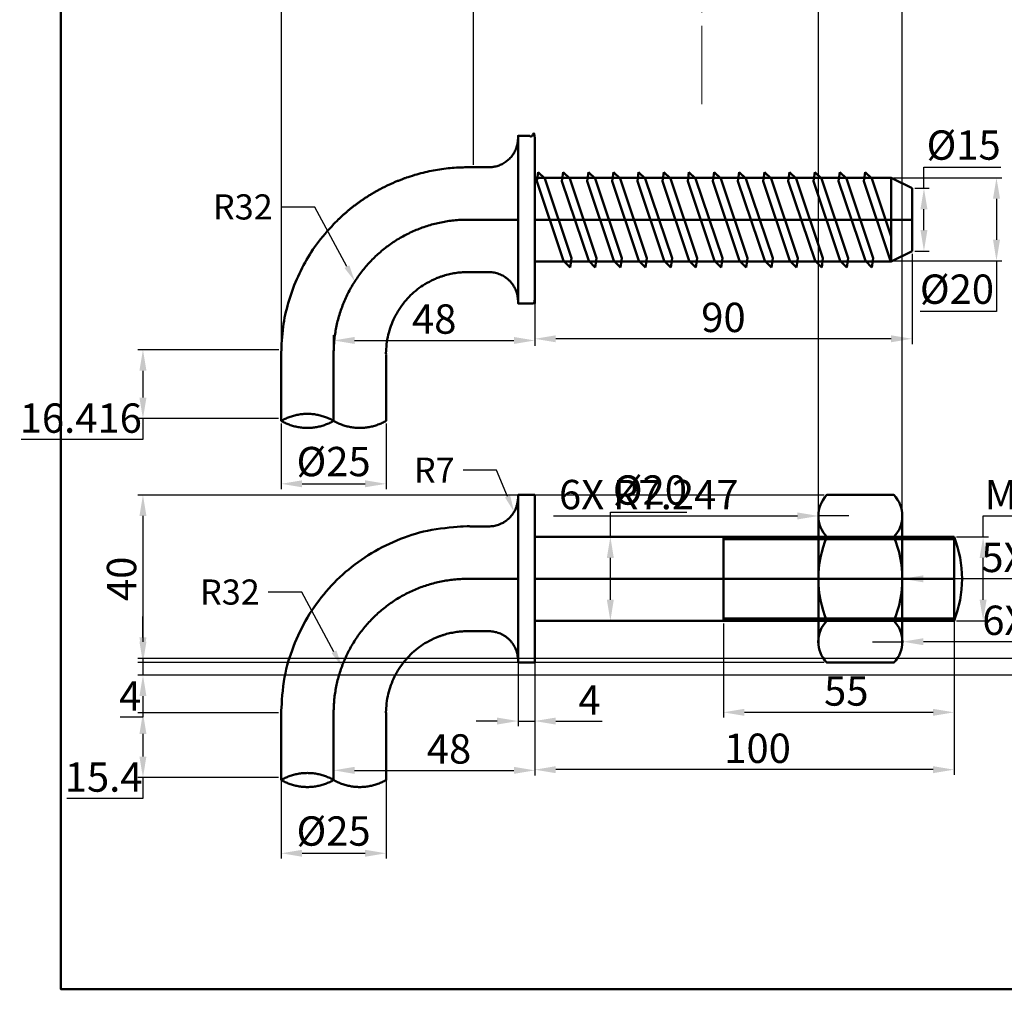
# Model space of a CAD drawing. Units: millimetres. Extents: x 120 to 482, y 299 to 766.
# Tile 1 of 3: x 120 to 355, y 299 to 531. Entities that reach past the tile are written whole.
import ezdxf
from ezdxf import colors
from ezdxf.entities.mleader import LeaderData, LeaderLine
from ezdxf.math import Vec2, Vec3

# ---------------------------------------------------------------- set-up
doc = ezdxf.new("R2010")
doc.units = ezdxf.units.MM
doc.linetypes.add('CENTER2', pattern=[28.575, 19.05, -3.175, 3.175, -3.175])
for name, color, linetype, lineweight in [('M-CNTR', 4, 'CENTER2', 18), ('M-DIMS', 2, 'Continuous', 25), ('M-OUTL', 7, 'Continuous', 50)]:
    doc.layers.add(name, color=color, linetype=linetype, lineweight=lineweight)
doc.styles.get("Standard").update_dxf_attribs({"font": 'arial.ttf'})
doc.dimstyles.new('ISO-25', dxfattribs={"dimtxt": 7, "dimasz": 5, "dimexe": 1.25, "dimexo": 0.625, "dimtad": 1, "dimtoh": 1, "dimdec": 0, "dimtxsty": 'Standard', "dimcen": 2.5, "dimadec": 0, "dimazin": 0, "dimtfac": 1, "dimtdec": 0, "dimtmove": 0, "dimatfit": 3, "dimfxl": 1, "dimarcsym": 0})

# ---------------------------------------------------------------- blocks, each defined once
blk = doc.blocks.new('*D1')
at = {"layer": 'Defpoints', "color": 0, "transparency": 16777216}
for p in [(182.11, 359.39), (207.11, 359.39), (207.11, 331.75)]:
    blk.add_point(p, dxfattribs=at)
at = {"layer": 'M-DIMS', "color": 0, "lineweight": -2, "transparency": 16777216}
for p, q in [((182.11, 358.77), (182.11, 330.5)), ((207.11, 358.77), (207.11, 330.5)), ((187.11, 331.75), (202.11, 331.75))]:
    blk.add_line(p, q, dxfattribs=at)
at = {"layer": 'M-DIMS', "color": 0, "transparency": 16777216}
for points in [[(187.11, 332.58), (187.11, 330.92), (182.11, 331.75)], [(202.11, 332.58), (202.11, 330.92), (207.11, 331.75)]]:
    blk.add_solid(points, dxfattribs=at)
at = {"layer": 'M-DIMS', "color": 0, "transparency": 16777216, "insert": (194.61, 336.15), "char_height": 7, "attachment_point": 5}
blk.add_mtext('%%C25', dxfattribs=at)
blk = doc.blocks.new('*D2')
at = {"layer": 'Defpoints', "color": 0, "transparency": 16777216}
for p in [(238.61, 412.32), (242.61, 412.32), (242.61, 363.3)]:
    blk.add_point(p, dxfattribs=at)
at = {"layer": 'M-DIMS', "color": 0, "lineweight": -2, "transparency": 16777216}
for p, q in [((238.61, 411.69), (238.61, 362.05)), ((242.61, 411.69), (242.61, 362.05)), ((233.61, 363.3), (228.61, 363.3)), ((238.61, 363.3), (242.61, 363.3)), ((247.61, 363.3), (258.7, 363.3))]:
    blk.add_line(p, q, dxfattribs=at)
at = {"layer": 'M-DIMS', "color": 0, "transparency": 16777216}
for points in [[(233.61, 364.13), (233.61, 362.46), (238.61, 363.3)], [(247.61, 364.13), (247.61, 362.46), (242.61, 363.3)]]:
    blk.add_solid(points, dxfattribs=at)
at = {"layer": 'M-DIMS', "color": 0, "transparency": 16777216, "insert": (255.66, 367.42), "char_height": 7, "attachment_point": 5}
blk.add_mtext('4', dxfattribs=at)
blk = doc.blocks.new('*D3')
at = {"layer": 'Defpoints', "color": 0, "transparency": 16777216}
for p in [(342.61, 407.23), (342.61, 387.23), (349.55, 387.23)]:
    blk.add_point(p, dxfattribs=at)
at = {"layer": 'M-DIMS', "color": 0, "lineweight": -2, "transparency": 16777216}
for p, q in [((349.55, 407.23), (349.55, 412.23)), ((349.55, 412.23), (368, 412.23)), ((343.23, 407.23), (350.8, 407.23)), ((349.55, 392.23), (349.55, 402.23)), ((343.23, 387.23), (350.8, 387.23))]:
    blk.add_line(p, q, dxfattribs=at)
at = {"layer": 'M-DIMS', "color": 0, "transparency": 16777216}
for points in [[(348.72, 402.23), (350.38, 402.23), (349.55, 407.23)], [(348.72, 392.23), (350.38, 392.23), (349.55, 387.23)]]:
    blk.add_solid(points, dxfattribs=at)
at = {"layer": 'M-DIMS', "color": 0, "transparency": 16777216, "insert": (359.09, 416.43), "char_height": 7, "attachment_point": 5}
blk.add_mtext('M20', dxfattribs=at)
blk = doc.blocks.new('*D4')
at = {"layer": 'Defpoints', "color": 0, "transparency": 16777216}
for p in [(287.61, 387.23), (342.61, 387.23), (342.61, 365.38)]:
    blk.add_point(p, dxfattribs=at)
at = {"layer": 'M-DIMS', "color": 0, "lineweight": -2, "transparency": 16777216}
for p, q in [((287.61, 386.61), (287.61, 364.13)), ((342.61, 386.61), (342.61, 364.13)), ((292.61, 365.38), (337.61, 365.38))]:
    blk.add_line(p, q, dxfattribs=at)
at = {"layer": 'M-DIMS', "color": 0, "transparency": 16777216}
for points in [[(292.61, 366.21), (292.61, 364.54), (287.61, 365.38)], [(337.61, 366.21), (337.61, 364.54), (342.61, 365.38)]]:
    blk.add_solid(points, dxfattribs=at)
at = {"layer": 'M-DIMS', "color": 0, "transparency": 16777216, "insert": (316.91, 369.56), "char_height": 7, "attachment_point": 5}
blk.add_mtext('55', dxfattribs=at)
blk = doc.blocks.new('*D5')
at = {"layer": 'Defpoints', "color": 0, "transparency": 16777216}
for p in [(342.61, 397.23), (242.61, 381.65), (242.61, 351.7)]:
    blk.add_point(p, dxfattribs=at)
at = {"layer": 'M-DIMS', "color": 0, "lineweight": -2, "transparency": 16777216}
for p, q in [((342.61, 396.61), (342.61, 350.45)), ((242.61, 381.03), (242.61, 350.45)), ((337.61, 351.7), (247.61, 351.7))]:
    blk.add_line(p, q, dxfattribs=at)
at = {"layer": 'M-DIMS', "color": 0, "transparency": 16777216}
for points in [[(247.61, 352.53), (247.61, 350.86), (242.61, 351.7)], [(337.61, 352.53), (337.61, 350.86), (342.61, 351.7)]]:
    blk.add_solid(points, dxfattribs=at)
at = {"layer": 'M-DIMS', "color": 0, "transparency": 16777216, "insert": (295.75, 355.9), "char_height": 7, "attachment_point": 5}
blk.add_mtext('100', dxfattribs=at)
blk = doc.blocks.new('*D6')
at = {"layer": 'Defpoints', "color": 0, "transparency": 16777216}
for p in [(242.61, 381.65), (194.61, 359.39), (242.61, 351.54)]:
    blk.add_point(p, dxfattribs=at)
at = {"layer": 'M-DIMS', "color": 0, "lineweight": -2, "transparency": 16777216}
for p, q in [((242.61, 381.03), (242.61, 350.29)), ((194.61, 358.77), (194.61, 350.29)), ((199.61, 351.54), (237.61, 351.54))]:
    blk.add_line(p, q, dxfattribs=at)
at = {"layer": 'M-DIMS', "color": 0, "transparency": 16777216}
for points in [[(199.61, 352.37), (199.61, 350.7), (194.61, 351.54)], [(237.61, 352.37), (237.61, 350.7), (242.61, 351.54)]]:
    blk.add_solid(points, dxfattribs=at)
at = {"layer": 'M-DIMS', "color": 0, "transparency": 16777216, "insert": (222.14, 355.74), "char_height": 7, "attachment_point": 5}
blk.add_mtext('48', dxfattribs=at)
blk = doc.blocks.new('*D7')
at = {"layer": 'Defpoints', "color": 0, "transparency": 16777216}
for p in [(182.11, 434.92), (207.11, 434.92), (207.11, 419.9)]:
    blk.add_point(p, dxfattribs=at)
at = {"layer": 'M-DIMS', "color": 0, "lineweight": -2, "transparency": 16777216}
for p, q in [((182.11, 434.29), (182.11, 418.65)), ((207.11, 434.29), (207.11, 418.65)), ((187.11, 419.9), (202.11, 419.9))]:
    blk.add_line(p, q, dxfattribs=at)
at = {"layer": 'M-DIMS', "color": 0, "transparency": 16777216}
for points in [[(187.11, 420.74), (187.11, 419.07), (182.11, 419.9)], [(202.11, 420.74), (202.11, 419.07), (207.11, 419.9)]]:
    blk.add_solid(points, dxfattribs=at)
at = {"layer": 'M-DIMS', "color": 0, "transparency": 16777216, "insert": (194.61, 424.3), "char_height": 7, "attachment_point": 5}
blk.add_mtext('%%C25', dxfattribs=at)
blk = doc.blocks.new('*D8')
at = {"layer": 'Defpoints', "color": 0, "transparency": 16777216}
for p in [(276.59, 407.23), (260.63, 387.23), (276.59, 387.23)]:
    blk.add_point(p, dxfattribs=at)
at = {"layer": 'M-DIMS', "color": 0, "lineweight": -2, "transparency": 16777216}
for p, q in [((260.63, 407.23), (260.63, 413.12)), ((260.63, 413.12), (278.87, 413.12)), ((275.96, 407.23), (259.38, 407.23)), ((260.63, 392.23), (260.63, 402.23)), ((275.96, 387.23), (259.38, 387.23))]:
    blk.add_line(p, q, dxfattribs=at)
at = {"layer": 'M-DIMS', "color": 0, "transparency": 16777216}
for points in [[(259.8, 402.23), (261.46, 402.23), (260.63, 407.23)], [(259.8, 392.23), (261.46, 392.23), (260.63, 387.23)]]:
    blk.add_solid(points, dxfattribs=at)
at = {"layer": 'M-DIMS', "color": 0, "transparency": 16777216, "insert": (270.06, 417.51), "char_height": 7, "attachment_point": 5}
blk.add_mtext('%%C20', dxfattribs=at)
blk = doc.blocks.new('*D9')
at = {"layer": 'Defpoints', "color": 0, "transparency": 16777216}
for p in [(332.61, 490.42), (332.61, 475.42), (335.44, 475.42)]:
    blk.add_point(p, dxfattribs=at)
at = {"layer": 'M-DIMS', "color": 0, "lineweight": -2, "transparency": 16777216}
for p, q in [((335.44, 490.42), (335.44, 495.42)), ((335.44, 495.42), (353.76, 495.42)), ((333.23, 490.42), (336.69, 490.42)), ((335.44, 480.42), (335.44, 485.42)), ((333.23, 475.42), (336.69, 475.42))]:
    blk.add_line(p, q, dxfattribs=at)
at = {"layer": 'M-DIMS', "color": 0, "transparency": 16777216}
for points in [[(334.61, 485.42), (336.27, 485.42), (335.44, 490.42)], [(334.61, 480.42), (336.27, 480.42), (335.44, 475.42)]]:
    blk.add_solid(points, dxfattribs=at)
at = {"layer": 'M-DIMS', "color": 0, "transparency": 16777216, "insert": (344.91, 499.81), "char_height": 7, "attachment_point": 5}
blk.add_mtext('%%C15', dxfattribs=at)
blk = doc.blocks.new('*D10')
at = {"layer": 'Defpoints', "color": 0, "transparency": 16777216}
for p in [(327.56, 492.92), (327.46, 473.12), (352.74, 473.12)]:
    blk.add_point(p, dxfattribs=at)
at = {"layer": 'M-DIMS', "color": 0, "lineweight": -2, "transparency": 16777216}
for p, q in [((328.18, 492.92), (353.99, 492.92)), ((352.74, 487.92), (352.74, 478.12)), ((328.08, 473.12), (353.99, 473.12)), ((352.74, 473.12), (352.74, 461.03)), ((352.74, 461.03), (334.5, 461.03))]:
    blk.add_line(p, q, dxfattribs=at)
at = {"layer": 'M-DIMS', "color": 0, "transparency": 16777216}
for points in [[(351.91, 487.92), (353.58, 487.92), (352.74, 492.92)], [(351.91, 478.12), (353.58, 478.12), (352.74, 473.12)]]:
    blk.add_solid(points, dxfattribs=at)
at = {"layer": 'M-DIMS', "color": 0, "transparency": 16777216, "insert": (343.31, 465.43), "char_height": 7, "attachment_point": 5}
blk.add_mtext('%%C20', dxfattribs=at)
blk = doc.blocks.new('*D11')
at = {"layer": 'Defpoints', "color": 0, "transparency": 16777216}
for p in [(332.61, 475.42), (242.61, 466.91), (242.61, 454.5)]:
    blk.add_point(p, dxfattribs=at)
at = {"layer": 'M-DIMS', "color": 0, "lineweight": -2, "transparency": 16777216}
for p, q in [((332.61, 474.79), (332.61, 453.25)), ((242.61, 466.28), (242.61, 453.25)), ((327.61, 454.5), (247.61, 454.5))]:
    blk.add_line(p, q, dxfattribs=at)
at = {"layer": 'M-DIMS', "color": 0, "transparency": 16777216}
for points in [[(247.61, 455.33), (247.61, 453.67), (242.61, 454.5)], [(327.61, 455.33), (327.61, 453.67), (332.61, 454.5)]]:
    blk.add_solid(points, dxfattribs=at)
at = {"layer": 'M-DIMS', "color": 0, "transparency": 16777216, "insert": (287.61, 458.7), "char_height": 7, "attachment_point": 5}
blk.add_mtext('90', dxfattribs=at)
blk = doc.blocks.new('*D12')
at = {"layer": 'Defpoints', "color": 0, "transparency": 16777216}
for p in [(242.61, 454.5), (242.61, 454.1), (194.61, 444.51)]:
    blk.add_point(p, dxfattribs=at)
at = {"layer": 'M-DIMS', "color": 0, "lineweight": -2, "transparency": 16777216}
for p, q in [((194.61, 445.13), (194.61, 455.35)), ((199.61, 454.1), (237.61, 454.1)), ((242.61, 453.88), (242.61, 452.85))]:
    blk.add_line(p, q, dxfattribs=at)
at = {"layer": 'M-DIMS', "color": 0, "transparency": 16777216}
for points in [[(199.61, 454.93), (199.61, 453.27), (194.61, 454.1)], [(237.61, 454.93), (237.61, 453.27), (242.61, 454.1)]]:
    blk.add_solid(points, dxfattribs=at)
at = {"layer": 'M-DIMS', "color": 0, "transparency": 16777216, "insert": (218.61, 458.3), "char_height": 7, "attachment_point": 5}
blk.add_mtext('48', dxfattribs=at)
blk = doc.blocks.new('*D37')
at = {"layer": 'Defpoints', "color": 0, "transparency": 16777216}
for p in [(228.01, 722.69), (228.01, 495.42), (182.15, 451.89)]:
    blk.add_point(p, dxfattribs=at)
at = {"layer": 'M-DIMS', "color": 0, "lineweight": -2, "transparency": 16777216}
for p, q in [((182.15, 452.51), (182.15, 723.94)), ((228.01, 496.04), (228.01, 723.94)), ((187.15, 722.69), (223.01, 722.69))]:
    blk.add_line(p, q, dxfattribs=at)
at = {"layer": 'M-DIMS', "color": 0, "transparency": 16777216}
for points in [[(187.15, 723.52), (187.15, 721.85), (182.15, 722.69)], [(223.01, 723.52), (223.01, 721.85), (228.01, 722.69)]]:
    blk.add_solid(points, dxfattribs=at)
at = {"layer": 'M-DIMS', "color": 0, "transparency": 16777216, "insert": (205.08, 726.89), "char_height": 7, "attachment_point": 5}
blk.add_mtext('45.86', dxfattribs=at)
blk = doc.blocks.new('*D38')
at = {"layer": 'Defpoints', "color": 0, "transparency": 16777216}
for p in [(182.15, 451.89), (149.13, 435.47), (182.11, 435.47)]:
    blk.add_point(p, dxfattribs=at)
at = {"layer": 'M-DIMS', "color": 0, "lineweight": -2, "transparency": 16777216}
for p, q in [((181.52, 451.89), (147.88, 451.89)), ((149.13, 446.89), (149.13, 440.47)), ((181.48, 435.47), (147.88, 435.47)), ((149.13, 435.47), (149.13, 430.47)), ((149.13, 430.47), (120.11, 430.47))]:
    blk.add_line(p, q, dxfattribs=at)
at = {"layer": 'M-DIMS', "color": 0, "transparency": 16777216}
for points in [[(148.29, 446.89), (149.96, 446.89), (149.13, 451.89)], [(148.29, 440.47), (149.96, 440.47), (149.13, 435.47)]]:
    blk.add_solid(points, dxfattribs=at)
at = {"layer": 'M-DIMS', "color": 0, "transparency": 16777216, "insert": (134.3, 434.67), "char_height": 7, "attachment_point": 5}
blk.add_mtext('16.416', dxfattribs=at)
blk = doc.blocks.new('*D39')
at = {"layer": 'Defpoints', "color": 0, "transparency": 16777216}
for p in [(182.11, 365.23), (149.13, 349.83), (182.11, 349.83)]:
    blk.add_point(p, dxfattribs=at)
at = {"layer": 'M-DIMS', "color": 0, "lineweight": -2, "transparency": 16777216}
for p, q in [((181.48, 365.23), (147.88, 365.23)), ((149.13, 360.23), (149.13, 354.83)), ((181.48, 349.83), (147.88, 349.83)), ((149.13, 349.83), (149.13, 344.83)), ((149.13, 344.83), (131.01, 344.83))]:
    blk.add_line(p, q, dxfattribs=at)
at = {"layer": 'M-DIMS', "color": 0, "transparency": 16777216}
for points in [[(148.29, 360.23), (149.96, 360.23), (149.13, 365.23)], [(148.29, 354.83), (149.96, 354.83), (149.13, 349.83)]]:
    blk.add_solid(points, dxfattribs=at)
at = {"layer": 'M-DIMS', "color": 0, "transparency": 16777216, "insert": (139.75, 349.03), "char_height": 7, "attachment_point": 5}
blk.add_mtext('15.4', dxfattribs=at)
blk = doc.blocks.new('*D40')
at = {"layer": 'Defpoints', "color": 0, "transparency": 16777216}
for p in [(312.27, 417.23), (149.13, 377.23), (312.27, 377.23)]:
    blk.add_point(p, dxfattribs=at)
at = {"layer": 'M-DIMS', "color": 0, "lineweight": -2, "transparency": 16777216}
for p, q in [((311.64, 417.23), (147.88, 417.23)), ((149.13, 412.23), (149.13, 382.23)), ((311.64, 377.23), (147.88, 377.23))]:
    blk.add_line(p, q, dxfattribs=at)
at = {"layer": 'M-DIMS', "color": 0, "transparency": 16777216}
for points in [[(148.29, 412.23), (149.96, 412.23), (149.13, 417.23)], [(148.29, 382.23), (149.96, 382.23), (149.13, 377.23)]]:
    blk.add_solid(points, dxfattribs=at)
at = {"layer": 'M-DIMS', "color": 0, "transparency": 16777216, "insert": (144.93, 397.23), "char_height": 7, "attachment_point": 5, "rotation": 90}
blk.add_mtext('40', dxfattribs=at)
blk = doc.blocks.new('*D41')
at = {"layer": 'Defpoints', "color": 0, "transparency": 16777216}
for p in [(330.27, 722.69), (310.27, 412.23), (330.27, 412.23)]:
    blk.add_point(p, dxfattribs=at)
at = {"layer": 'M-DIMS', "color": 0, "lineweight": -2, "transparency": 16777216}
for p, q in [((310.27, 412.86), (310.27, 723.94)), ((330.27, 412.86), (330.27, 723.94)), ((315.27, 722.69), (325.27, 722.69))]:
    blk.add_line(p, q, dxfattribs=at)
at = {"layer": 'M-DIMS', "color": 0, "transparency": 16777216}
for points in [[(315.27, 723.52), (315.27, 721.85), (310.27, 722.69)], [(325.27, 723.52), (325.27, 721.85), (330.27, 722.69)]]:
    blk.add_solid(points, dxfattribs=at)
at = {"layer": 'M-DIMS', "color": 0, "transparency": 16777216, "insert": (320.27, 726.89), "char_height": 7, "attachment_point": 5}
blk.add_mtext('20', dxfattribs=at)
blk = doc.blocks.new('*D42')
at = {"layer": 'Defpoints', "color": 0, "transparency": 16777216}
for p in [(376.62, 378.25), (149.13, 374.25), (376.62, 374.25)]:
    blk.add_point(p, dxfattribs=at)
at = {"layer": 'M-DIMS', "color": 0, "lineweight": -2, "transparency": 16777216}
for p, q in [((149.13, 383.25), (149.13, 388.25)), ((376, 378.25), (147.88, 378.25)), ((149.13, 378.25), (149.13, 374.25)), ((376, 374.25), (147.88, 374.25)), ((149.13, 369.25), (149.13, 364.25)), ((149.13, 364.25), (143.66, 364.25))]:
    blk.add_line(p, q, dxfattribs=at)
at = {"layer": 'M-DIMS', "color": 0, "transparency": 16777216}
for points in [[(148.29, 383.25), (149.96, 383.25), (149.13, 378.25)], [(148.29, 369.25), (149.96, 369.25), (149.13, 374.25)]]:
    blk.add_solid(points, dxfattribs=at)
at = {"layer": 'M-DIMS', "color": 0, "transparency": 16777216, "insert": (146.08, 368.37), "char_height": 7, "attachment_point": 5}
blk.add_mtext('4', dxfattribs=at)
blk = doc.blocks.new('*D44')
at = {"layer": 'Defpoints', "color": 0, "transparency": 16777216}
for p in [(304.27, 397.23), (330.27, 397.23)]:
    blk.add_point(p, dxfattribs=at)
at = {"layer": 'M-DIMS', "color": 0, "lineweight": -2, "transparency": 16777216}
for p, q in [((304.27, 397.23), (330.27, 397.23)), ((347.42, 397.23), (335.27, 397.23)), ((379.8, 397.23), (347.42, 397.23))]:
    blk.add_line(p, q, dxfattribs=at)
at = {"layer": 'M-DIMS', "color": 0, "transparency": 16777216}
blk.add_solid([(335.27, 398.06), (335.27, 396.4), (330.27, 397.23)], dxfattribs=at)
at = {"layer": 'M-DIMS', "color": 0, "transparency": 16777216, "insert": (363.92, 401.43), "char_height": 7, "attachment_point": 5}
blk.add_mtext('5X R26', dxfattribs=at)
blk = doc.blocks.new('*D45')
at = {"layer": 'Defpoints', "color": 0, "transparency": 16777216}
for p in [(310.27, 412.23), (317.52, 412.23)]:
    blk.add_point(p, dxfattribs=at)
at = {"layer": 'M-DIMS', "color": 0, "lineweight": -2, "transparency": 16777216}
for p, q in [((247.09, 412.23), (293.12, 412.23)), ((293.12, 412.23), (305.27, 412.23)), ((317.52, 412.23), (310.27, 412.23))]:
    blk.add_line(p, q, dxfattribs=at)
at = {"layer": 'M-DIMS', "color": 0, "transparency": 16777216}
blk.add_solid([(305.27, 413.06), (305.27, 411.4), (310.27, 412.23)], dxfattribs=at)
at = {"layer": 'M-DIMS', "color": 0, "transparency": 16777216, "insert": (269.79, 416.43), "char_height": 7, "attachment_point": 5}
blk.add_mtext('6X R7.247', dxfattribs=at)
blk = doc.blocks.new('*D46')
at = {"layer": 'Defpoints', "color": 0, "transparency": 16777216}
for p in [(323.14, 382.23), (330.3, 382.23)]:
    blk.add_point(p, dxfattribs=at)
at = {"layer": 'M-DIMS', "color": 0, "lineweight": -2, "transparency": 16777216}
for p, q in [((323.14, 382.23), (330.3, 382.23)), ((347.45, 382.23), (335.3, 382.23)), ((393.45, 382.23), (347.45, 382.23))]:
    blk.add_line(p, q, dxfattribs=at)
at = {"layer": 'M-DIMS', "color": 0, "transparency": 16777216}
blk.add_solid([(335.3, 383.06), (335.3, 381.4), (330.3, 382.23)], dxfattribs=at)
at = {"layer": 'M-DIMS', "color": 0, "transparency": 16777216, "insert": (370.76, 386.43), "char_height": 7, "attachment_point": 5}
blk.add_mtext('6X R7.164', dxfattribs=at)

msp = doc.modelspace()

# ---------------------------------------------------------------- linework, layer by layer
at = {"layer": 'M-CNTR'}
msp.add_line((282.4211, 700.5865), (282.4211, 510.4949), dxfattribs=at)
at = {"layer": 'M-OUTL'}
for p, q in [((243.383, 494.2888), (243.0736, 492.0742)), ((243.383, 494.2888), (244.969, 492.7125)), ((249.383, 494.2888), (249.0736, 492.0742)), ((249.383, 494.2888), (250.969, 492.7125)), ((255.383, 494.2888), (255.0736, 492.0742)), ((255.383, 494.2888), (256.969, 492.7125)), ((261.383, 494.2888), (261.0736, 492.0742)), ((261.383, 494.2888), (262.969, 492.7125)), ((267.383, 494.2888), (267.0736, 492.0742)), ((267.383, 494.2888), (268.969, 492.7125)), ((273.383, 494.2888), (273.0736, 492.0742)), ((273.383, 494.2888), (274.969, 492.7125)), ((279.383, 494.2888), (279.0736, 492.0742)), ((279.383, 494.2888), (280.969, 492.7125)), ((285.383, 494.2888), (285.0736, 492.0742)), ((285.383, 494.2888), (286.969, 492.7125)), ((291.383, 494.2888), (291.0736, 492.0742)), ((291.383, 494.2888), (292.969, 492.7125)), ((297.383, 494.2888), (297.0736, 492.0742)), ((297.383, 494.2888), (298.969, 492.7125)), ((303.383, 494.2888), (303.0736, 492.0742)), ((303.383, 494.2888), (304.969, 492.7125)), ((309.383, 494.2888), (309.0736, 492.0742)), ((309.383, 494.2888), (310.969, 492.7125)), ((315.383, 494.2888), (315.0736, 492.0742)), ((315.383, 494.2888), (316.969, 492.7125)), ((321.383, 494.2888), (321.0736, 492.0742)), ((321.383, 494.2888), (322.969, 492.7125)), ((243.0736, 492.0742), (249.4564, 473.1201)), ((251.3518, 473.7584), (244.969, 492.7125)), ((249.0736, 492.0742), (255.4564, 473.1201)), ((257.3518, 473.7584), (250.969, 492.7125)), ((255.0736, 492.0742), (261.4564, 473.1201)), ((263.3518, 473.7584), (256.969, 492.7125)), ((261.0736, 492.0742), (267.4564, 473.1201)), ((269.3518, 473.7584), (262.969, 492.7125)), ((267.0736, 492.0742), (273.4564, 473.1201)), ((275.3518, 473.7584), (268.969, 492.7125)), ((273.0736, 492.0742), (279.4564, 473.1201)), ((281.3518, 473.7584), (274.969, 492.7125)), ((279.0736, 492.0742), (285.4564, 473.1201)), ((287.3518, 473.7584), (280.969, 492.7125)), ((285.0736, 492.0742), (291.4564, 473.1201)), ((293.3518, 473.7584), (286.969, 492.7125)), ((327.61, 492.9163), (287.61, 492.9163)), ((291.0736, 492.0742), (297.4564, 473.1201)), ((299.3518, 473.7584), (292.969, 492.7125)), ((297.0736, 492.0742), (303.4564, 473.1201)), ((305.3518, 473.7584), (298.969, 492.7125)), ((303.0736, 492.0742), (309.4564, 473.1201)), ((311.3518, 473.7584), (304.969, 492.7125)), ((309.0736, 492.0742), (315.4564, 473.1201)), ((317.3518, 473.7584), (310.969, 492.7125)), ((315.0736, 492.0742), (321.4564, 473.1201)), ((323.3518, 473.7584), (316.969, 492.7125)), ((321.0736, 492.0742), (327.4564, 473.1201)), ((327.61, 478.9309), (322.969, 492.7125)), ((327.61, 492.9163), (327.61, 472.9163)), ((327.61, 492.9163), (332.61, 490.4163)), ((332.61, 475.4163), (332.61, 490.4163)), ((327.61, 472.9163), (332.61, 475.4163)), ((251.0424, 471.5438), (249.4564, 473.1201)), ((251.0424, 471.5438), (251.3518, 473.7584)), ((257.0424, 471.5438), (255.4564, 473.1201)), ((257.0424, 471.5438), (257.3518, 473.7584)), ((263.0424, 471.5438), (261.4564, 473.1201)), ((263.0424, 471.5438), (263.3518, 473.7584)), ((269.0424, 471.5438), (267.4564, 473.1201)), ((269.0424, 471.5438), (269.3518, 473.7584)), ((275.0424, 471.5438), (273.4564, 473.1201)), ((275.0424, 471.5438), (275.3518, 473.7584)), ((281.0424, 471.5438), (279.4564, 473.1201)), ((281.0424, 471.5438), (281.3518, 473.7584)), ((287.0424, 471.5438), (285.4564, 473.1201)), ((287.0424, 471.5438), (287.3518, 473.7584)), ((293.0424, 471.5438), (291.4564, 473.1201)), ((293.0424, 471.5438), (293.3518, 473.7584)), ((299.0424, 471.5438), (297.4564, 473.1201)), ((299.0424, 471.5438), (299.3518, 473.7584)), ((305.0424, 471.5438), (303.4564, 473.1201)), ((305.0424, 471.5438), (305.3518, 473.7584)), ((311.0424, 471.5438), (309.4564, 473.1201)), ((311.0424, 471.5438), (311.3518, 473.7584)), ((312.2686, 472.9163), (327.6614, 472.9163)), ((317.0424, 471.5438), (315.4564, 473.1201)), ((317.0424, 471.5438), (317.3518, 473.7584)), ((323.0424, 471.5438), (321.4564, 473.1201)), ((323.0424, 471.5438), (323.3518, 473.7584)), ((327.6614, 472.9163), (327.4564, 473.1201)), ((329.3518, 473.7584), (329.3435, 473.7831)), ((310.2686, 412.3511), (310.2686, 381.5397)), ((330.2686, 381.5397), (330.2686, 412.3511)), ((287.61, 387.2311), (287.61, 407.2311)), ((287.61, 406.7311), (342.61, 406.7311)), ((330.2686, 407.2311), (312.2686, 407.2311)), ((342.61, 387.2311), (342.61, 407.2311)), ((287.61, 387.7311), (342.61, 387.7311)), ((312.2686, 387.2311), (328.2686, 387.2311))]:
    msp.add_line(p, q, dxfattribs=at)
msp.add_lwpolyline([(129.5751, 766.022), (472.9721, 766.022), (472.9721, 299.2966), (129.5751, 299.2966)], close=True, dxfattribs=at)
for points in [[(287.61, 492.9163), (242.61, 492.9163)], [(332.61, 482.9163), (242.61, 482.9163), (242.61, 462.9163)], [(242.61, 472.9163), (327.61, 472.9163)], [(342.61, 397.2311), (242.61, 397.2311), (242.61, 377.2311)]]:
    msp.add_lwpolyline(points, dxfattribs=at)
msp.add_lwpolyline([(312.2686, 407.2311, 0.2), (312.2686, 387.2311, 0.40668757), (312.2686, 377.2311), (328.2686, 377.2311, 0.40668757), (328.2686, 387.2311, 0.2), (328.2686, 407.2311, 0.40019879), (328.2686, 417.2311), (312.2686, 417.2311, 0.40019879)], format="xyb", close=True, dxfattribs=at)
msp.add_lwpolyline([(242.61, 387.2311), (342.61, 387.2311, 0.19274298), (342.61, 407.2311), (242.61, 407.2311)], format="xyb", dxfattribs=at)
for points, weights, knots in [([(238.61, 502.4163), (238.61, 489.4163), (238.61, 476.4163), (238.61, 463.4163), (238.61, 463.2496), (238.61, 463.083), (238.61, 462.9163), (239.9433, 462.9163), (241.2767, 462.9163), (242.61, 462.9163), (242.61, 476.2496), (242.61, 489.583), (242.61, 502.9163), (241.2767, 502.9163), (239.9433, 502.9163), (238.61, 502.9163), (238.61, 502.7496), (238.61, 502.583), (238.61, 502.4163), (238.61, 498.3158), (235.7105, 495.4163), (231.61, 495.4163), (229.9433, 495.4163), (228.2767, 495.4163), (226.61, 495.4163), (214.6501, 495.4163), (203.6006, 490.8395), (195.1437, 482.3826), (186.6868, 473.9257), (182.11, 462.8762), (182.11, 450.9163), (182.11, 448.9163), (182.11, 446.9163), (182.11, 444.9163), (182.11, 441.583), (182.11, 438.2496), (182.11, 434.9163)], [1, 1, 1, 1, 1, 1, 1, 1, 1, 1, 1, 1, 1, 1, 1, 1, 1, 1, 1, 0.804737854124, 0.804737854124, 1, 1, 1, 1, 0.949253021674, 0.949253021674, 1, 0.949253021674, 0.949253021674, 1, 1, 1, 1, 1, 1, 1], [0, 0, 0, 0, 1, 1, 1, 2, 2, 2, 3, 3, 3, 4, 4, 4, 5, 5, 5, 6, 6, 6, 7.57079633, 7.57079633, 7.57079633, 8.57079633, 8.57079633, 8.57079633, 9.35619449, 9.35619449, 9.35619449, 10.14159265, 10.14159265, 10.14159265, 16.14159265, 16.14159265, 16.14159265, 17.14159265, 17.14159265, 17.14159265, 17.14159265]), ([(194.61, 434.9163), (194.61, 440.2496), (194.61, 445.583), (194.61, 450.9163), (194.61, 459.5167), (197.9012, 467.4624), (203.9826, 473.5437), (210.0639, 479.6251), (218.0096, 482.9163), (226.61, 482.9163), (230.61, 482.9163), (234.61, 482.9163), (238.61, 482.9163)], [1, 1, 1, 1, 0.949253021674, 0.949253021674, 1, 0.949253021674, 0.949253021674, 1, 1, 1, 1], [14.28318531, 14.28318531, 14.28318531, 14.28318531, 15.28318531, 15.28318531, 15.28318531, 16.06858347, 16.06858347, 16.06858347, 16.85398163, 16.85398163, 16.85398163, 17.85398163, 17.85398163, 17.85398163, 17.85398163]), ([(238.61, 463.4163), (238.61, 467.5168), (235.7105, 470.4163), (231.61, 470.4163), (229.9433, 470.4163), (228.2767, 470.4163), (226.61, 470.4163), (221.3691, 470.4163), (216.5272, 468.4107), (212.8214, 464.7049), (209.1156, 460.9991), (207.11, 456.1572), (207.11, 450.9163), (207.11, 448.9163), (207.11, 446.9163), (207.11, 444.9163), (207.11, 441.583), (207.11, 438.2496), (207.11, 434.9163)], [1, 0.804737854124, 0.804737854124, 1, 1, 1, 1, 0.949253021674, 0.949253021674, 1, 0.949253021674, 0.949253021674, 1, 1, 1, 1, 1, 1, 1], [0, 0, 0, 0, 1.57079633, 1.57079633, 1.57079633, 2.57079633, 2.57079633, 2.57079633, 3.35619449, 3.35619449, 3.35619449, 4.14159265, 4.14159265, 4.14159265, 10.14159265, 10.14159265, 10.14159265, 11.14159265, 11.14159265, 11.14159265, 11.14159265]), ([(207.11, 434.9163), (203.1476, 432.6287), (198.5723, 432.6287), (194.61, 434.9163), (190.6476, 437.204), (186.0723, 437.204), (182.11, 434.9163)], [1, 0.910683602523, 0.910683602523, 1, 0.910683602523, 0.910683602523, 1], [11.14159265, 11.14159265, 11.14159265, 11.14159265, 12.1887902, 12.1887902, 12.1887902, 13.23598776, 13.23598776, 13.23598776, 13.23598776]), ([(238.61, 417.2311), (238.61, 417.0644), (238.61, 416.8978), (238.61, 416.7311), (238.61, 412.6306), (235.7105, 409.7311), (231.61, 409.7311), (229.9433, 409.7311), (228.2767, 409.7311), (226.61, 409.7311), (214.6501, 409.7311), (203.6006, 405.1542), (195.1437, 396.6973), (186.6868, 388.2404), (182.11, 377.191), (182.11, 365.2311), (182.11, 363.2311), (182.11, 361.2311), (182.11, 359.2311), (182.11, 355.8978), (182.11, 352.5644), (182.11, 349.2311)], [1, 1, 1, 1, 0.804737854124, 0.804737854124, 1, 1, 1, 1, 0.949253021674, 0.949253021674, 1, 0.949253021674, 0.949253021674, 1, 1, 1, 1, 1, 1, 1], [5, 5, 5, 5, 6, 6, 6, 7.57079633, 7.57079633, 7.57079633, 8.57079633, 8.57079633, 8.57079633, 9.35619449, 9.35619449, 9.35619449, 10.14159265, 10.14159265, 10.14159265, 16.14159265, 16.14159265, 16.14159265, 17.14159265, 17.14159265, 17.14159265, 17.14159265]), ([(194.61, 349.2311), (194.61, 354.5644), (194.61, 359.8978), (194.61, 365.2311), (194.61, 373.8314), (197.9012, 381.7771), (203.9826, 387.8585), (210.0639, 393.9399), (218.0096, 397.2311), (226.61, 397.2311), (230.61, 397.2311), (234.61, 397.2311), (238.61, 397.2311)], [1, 1, 1, 1, 0.949253021674, 0.949253021674, 1, 0.949253021674, 0.949253021674, 1, 1, 1, 1], [14.28318531, 14.28318531, 14.28318531, 14.28318531, 15.28318531, 15.28318531, 15.28318531, 16.06858347, 16.06858347, 16.06858347, 16.85398163, 16.85398163, 16.85398163, 17.85398163, 17.85398163, 17.85398163, 17.85398163]), ([(238.61, 377.7311), (238.61, 381.8316), (235.7105, 384.7311), (231.61, 384.7311), (229.9433, 384.7311), (228.2767, 384.7311), (226.61, 384.7311), (221.3691, 384.7311), (216.5272, 382.7255), (212.8214, 379.0197), (209.1156, 375.3138), (207.11, 370.4719), (207.11, 365.2311), (207.11, 363.2311), (207.11, 361.2311), (207.11, 359.2311), (207.11, 355.8978), (207.11, 352.5644), (207.11, 349.2311)], [1, 0.804737854124, 0.804737854124, 1, 1, 1, 1, 0.949253021674, 0.949253021674, 1, 0.949253021674, 0.949253021674, 1, 1, 1, 1, 1, 1, 1], [0, 0, 0, 0, 1.57079633, 1.57079633, 1.57079633, 2.57079633, 2.57079633, 2.57079633, 3.35619449, 3.35619449, 3.35619449, 4.14159265, 4.14159265, 4.14159265, 10.14159265, 10.14159265, 10.14159265, 11.14159265, 11.14159265, 11.14159265, 11.14159265]), ([(207.11, 349.2311), (203.1476, 346.9434), (198.5723, 346.9434), (194.61, 349.2311), (190.6476, 351.5187), (186.0723, 351.5187), (182.11, 349.2311)], [1, 0.910683602523, 0.910683602523, 1, 0.910683602523, 0.910683602523, 1], [11.14159265, 11.14159265, 11.14159265, 11.14159265, 12.1887902, 12.1887902, 12.1887902, 13.23598776, 13.23598776, 13.23598776, 13.23598776])]:
    msp.add_rational_spline(points, weights, degree=3, knots=knots, dxfattribs=at)
for points in [[(182.11, 434.9163), (186.0723, 432.6287), (190.6476, 432.6287), (194.61, 434.9163)], [(182.11, 349.2311), (186.0723, 346.9434), (190.6476, 346.9434), (194.61, 349.2311)]]:
    msp.add_rational_spline(points, [1, 0.910683602523, 0.910683602523, 1], degree=3, dxfattribs=at)
for points in [[(242.61, 417.2311), (241.2767, 417.2311), (239.9433, 417.2311), (238.61, 417.2311)], [(242.61, 377.2311), (242.61, 390.5644), (242.61, 403.8978), (242.61, 417.2311)], [(238.61, 377.2311), (239.9433, 377.2311), (241.2767, 377.2311), (242.61, 377.2311)]]:
    msp.add_open_spline(points, degree=3, dxfattribs=at)
msp.add_open_spline([(238.61, 416.7311), (238.61, 403.7311), (238.61, 390.7311), (238.61, 377.7311), (238.61, 377.5644), (238.61, 377.3978), (238.61, 377.2311)], degree=3, knots=[0, 0, 0, 0, 1, 1, 1, 2, 2, 2, 2], dxfattribs=at)

# ---------------------------------------------------------------- dimensions: what is measured, and where the dimension line sits
at = {"layer": 'M-DIMS'}
for base, p1, p2, override, picture, middle in [((228.0077, 722.6865), (182.1455, 451.8868), (228.0077, 495.4163), {"dimdec": 2, "dimlfac": 1, "dimrnd": 0, "dimzin": 0, "dimdsep": 46, "dimlunit": 2}, '*D37', (205.0766, 726.8855)), ((330.2696, 722.6865), (310.2676, 412.2311), (330.2696, 412.2311), {"dimdec": 0, "dimlfac": 1, "dimrnd": 0, "dimzin": 0, "dimdsep": 46, "dimlunit": 2}, '*D41', (320.2686, 726.8855)), ((242.61, 454.5014), (332.61, 475.4163), (242.61, 466.9098), {"dimclrd": 0, "dimclre": 0, "dimclrt": 0}, '*D11', (287.61, 458.7004)), ((242.61, 454.1016), (194.61, 444.5055), (242.61, 454.5014), {"dimclrd": 0, "dimclre": 0, "dimclrt": 0}, '*D12', (218.61, 458.3006)), ((242.61, 363.2955), (238.61, 412.3156), (242.61, 412.3156), {"dimclrd": 0, "dimclre": 0, "dimclrt": 0}, '*D2', (255.6559, 367.4205))]:
    dim = msp.add_linear_dim(base=base, p1=p1, p2=p2, dimstyle='ISO-25', override=override, dxfattribs=at)
    dim.commit()
    dim.dimension.update_dxf_attribs({"geometry": picture, "text_midpoint": middle})
for base, p1, p2, text, picture, middle in [((335.4409, 475.4163), (332.61, 490.4163), (332.61, 475.4163), '%%C<>', '*D9', (344.9138, 495.4163)), ((352.7431, 473.1201), (327.5589, 492.9163), (327.4564, 473.1201), '%%C<>', '*D10', (343.3084, 461.0332)), ((260.6285, 387.2311), (276.5855, 407.2311), (276.5855, 387.2311), '%%C<>', '*D8', (270.0632, 413.1169)), ((349.5499, 387.2311), (342.61, 407.2311), (342.61, 387.2311), 'M<>', '*D3', (359.0896, 412.2311))]:
    dim = msp.add_linear_dim(base=base, p1=p1, p2=p2, angle=90, text=text, dimstyle='ISO-25', override={"dimclrd": 0, "dimclre": 0, "dimclrt": 0}, dxfattribs=at)
    dim.commit()
    dim.dimension.update_dxf_attribs({"geometry": picture, "text_midpoint": middle, "dimtype": 160})
for base, p1, p2, override, picture, middle in [((149.1271, 435.4712), (182.1455, 451.8868), (182.11, 435.4712), {"dimdec": 3, "dimlfac": 1, "dimrnd": 0, "dimzin": 0, "dimdsep": 46, "dimlunit": 2}, '*D38', (134.3039, 434.6703)), ((149.1271, 377.2311), (312.2686, 417.2311), (312.2686, 377.2311), {"dimdec": 0, "dimlfac": 1, "dimrnd": 0, "dimzin": 0, "dimdsep": 46, "dimlunit": 2}, '*D40', (144.9281, 397.2311)), ((149.1271, 374.2458), (376.6246, 378.2458), (376.6246, 374.2458), {"dimdec": 0, "dimlfac": 1, "dimrnd": 0, "dimzin": 0, "dimdsep": 46, "dimlunit": 2}, '*D42', (146.0812, 368.3708)), ((149.1271, 349.8301), (182.11, 365.23), (182.11, 349.8301), {"dimdec": 1, "dimlfac": 1, "dimrnd": 0, "dimzin": 0, "dimdsep": 46, "dimlunit": 2}, '*D39', (139.7545, 349.0292))]:
    dim = msp.add_linear_dim(base=base, p1=p1, p2=p2, angle=90, dimstyle='ISO-25', override=override, dxfattribs=at)
    dim.commit()
    dim.dimension.update_dxf_attribs({"geometry": picture, "text_midpoint": middle})
for base, p1, p2, picture, middle in [((207.11, 419.9035), (182.11, 434.9163), (207.11, 434.9163), '*D7', (194.61, 424.2983)), ((207.11, 331.7517), (182.11, 359.3907), (207.11, 359.3907), '*D1', (194.61, 336.1464))]:
    dim = msp.add_linear_dim(base=base, p1=p1, p2=p2, text='%%C<>', dimstyle='ISO-25', override={"dimclrd": 0, "dimclre": 0, "dimclrt": 0}, dxfattribs=at)
    dim.commit()
    dim.dimension.update_dxf_attribs({"geometry": picture, "text_midpoint": middle})
for center, mpoint, text, override, picture, middle in [((317.515, 412.2311), (310.2676, 412.231), '6X <>', {"dimdec": 3, "dimlfac": 1, "dimrnd": 0, "dimzin": 0, "dimdsep": 46, "dimlunit": 2}, '*D45', (269.7947, 416.4298)), ((304.2686, 397.2311), (330.2686, 397.231), '5X <>', {"dimdec": 0, "dimlfac": 1, "dimrnd": 0, "dimzin": 0, "dimdsep": 46, "dimlunit": 2}, '*D44', (363.9229, 401.43)), ((323.1381, 382.2311), (330.302, 382.231), '6X <>', {"dimdec": 3, "dimlfac": 1, "dimrnd": 0, "dimzin": 0, "dimdsep": 46, "dimlunit": 2}, '*D46', (370.7606, 386.4298))]:
    dim = msp.add_radius_dim(center=center, mpoint=mpoint, text=text, dimstyle='ISO-25', override=override, dxfattribs=at)
    dim.commit()
    dim.dimension.update_dxf_attribs({"geometry": picture, "text_midpoint": middle})
for base, p1, p2, picture, middle in [((242.61, 351.6971), (342.61, 397.2311), (242.61, 381.6511), '*D5', (295.7528, 351.6971)), ((342.61, 365.3768), (287.61, 387.2311), (342.61, 387.2311), '*D4', (316.9092, 365.3768)), ((242.61, 351.536), (194.61, 359.3907), (242.61, 381.6511), '*D6', (222.1384, 351.536))]:
    dim = msp.add_linear_dim(base=base, p1=p1, p2=p2, dimstyle='ISO-25', override={"dimclrd": 0, "dimclre": 0, "dimclrt": 0}, dxfattribs=at)
    dim.commit()
    dim.dimension.update_dxf_attribs({"geometry": picture, "text_midpoint": middle, "dimtype": 160})

# ---------------------------------------------------------------- leaders
ml = msp.add_multileader_mtext('Standard', dxfattribs=at)
ml.set_content('R32', color=256)
ml.set_leader_properties()
ml.build(insert=Vec2(0, 0))
ctx = ml.context
ctx.base_point, ctx.char_height, ctx.plane_origin = Vec3(163.8226, 485.9099), 6, Vec3(199.6809, 468.2029)
ctx.text_align_type = 2
notes = []
notes.append((ctx, [(0, (1, 1, 0), (190.0981, 485.9099), (-1, 0), 8, [(0, [(199.6809, 468.2029)], 0, [])])]))
ctx.mtext.insert, ctx.mtext.alignment, ctx.mtext.flow_direction = Vec3(180.0981, 488.9631), 3, 5
ml = msp.add_multileader_mtext('Standard', dxfattribs=at)
ml.set_content('R7', color=256)
ml.set_leader_properties()
ml.build(insert=Vec2(0, 0))
ctx = ml.context
ctx.base_point, ctx.char_height, ctx.plane_origin = Vec3(211.8284, 423.1601), 6, Vec3(237.6566, 413.2042)
ctx.text_align_type = 2
notes.append((ctx, [(0, (1, 1, 0), (233.5037, 423.1601), (-1, 0), 8, [(0, [(237.6566, 413.2042)], 0, [])])]))
ctx.mtext.insert, ctx.mtext.alignment, ctx.mtext.flow_direction = Vec3(223.5037, 426.1601), 3, 5
ml = msp.add_multileader_mtext('Standard', dxfattribs=at)
ml.set_content('R32', color=256)
ml.set_leader_properties()
ml.build(insert=Vec2(0, 0))
ctx = ml.context
ctx.base_point, ctx.char_height, ctx.plane_origin = Vec3(160.7344, 394.0272), 6, Vec3(196.5928, 376.3201)
ctx.text_align_type = 2
notes.append((ctx, [(0, (1, 1, 0), (187.01, 394.0272), (-1, 0), 8, [(0, [(196.5928, 376.3201)], 0, [])])]))
ctx.mtext.insert, ctx.mtext.alignment, ctx.mtext.flow_direction = Vec3(177.01, 397.0804), 3, 5
for ctx, leaders in notes:
    for number, flags, end, landing, length, lines in leaders:
        leader = LeaderData()
        leader.index, (leader.has_last_leader_line, leader.has_dogleg_vector, leader.attachment_direction) = number, flags
        leader.last_leader_point, leader.dogleg_vector, leader.dogleg_length = Vec3(end), Vec3(landing), length
        for number, points, colour, breaks in lines:
            line = LeaderLine()
            line.index, line.vertices, line.color, line.breaks = number, Vec3.list(points), colors.encode_raw_color(colour), breaks
            leader.lines.append(line)
        ctx.leaders.append(leader)

doc.saveas('drawing.dxf')
